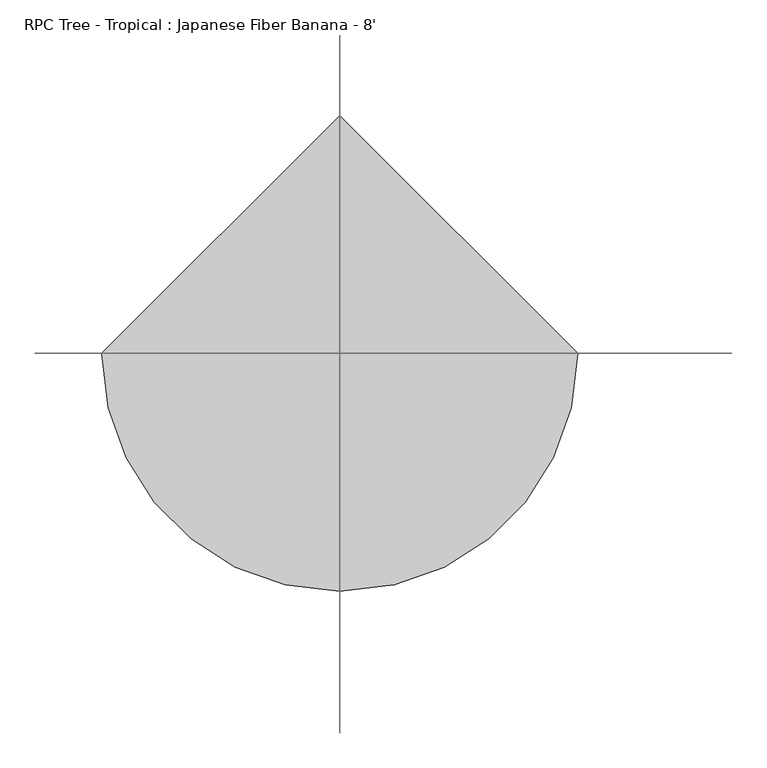
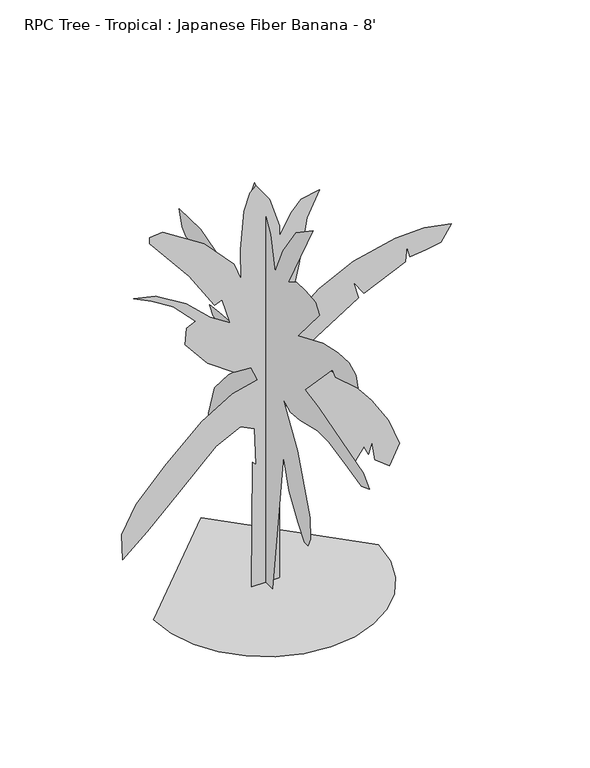
"""IFC4 building model written with IfcOpenShell, lengths in millimetres: geographic element geometry, RPC Tree - Tropical : Japanese Fiber Banana - 8'."""

from ifc_helpers import new_model, si_unit, origin, place, context, project, spatial, triangles, source, transform, mapped, element, save


def rpc_tree_tropical_japanese_fiber_banana_8_fc2fb2a9(model_context):
    return source(origin(), model_context, "Body", "Tessellation", [
        triangles([(-649.7467501, 0.0, 3.7e-06), (-632.5712723, -148.8792756, 3.7e-06), (-583.6506755, -285.6010629, 3.7e-06), (-506.9043426, -406.2488949, 3.7e-06), (-406.2488949, -506.9043426, 3.7e-06), (-285.6010629, -583.6506755, 3.7e-06), (-148.8792756, -632.5712723, 3.7e-06), (2.84e-05, -649.7467501, 3.7e-06), (148.8792756, -632.5712723, 3.7e-06), (285.6010629, -583.6506755, 3.7e-06), (406.2488949, -506.9043426, 3.7e-06), (506.9043426, -406.2488949, 3.7e-06), (583.6506755, -285.6010629, 3.7e-06), (632.5712723, -148.8790212, 3.7e-06), (649.7467501, 5.68e-05, 3.7e-06), (-8.52e-05, 649.7467501, 3.7e-06), (73.5169788, -2.4e-06, 1488.9400761), (86.1999983, -4e-06, 1501.9626823), (108.3956093, -6.3e-06, 1521.7797867), (138.5178168, -9.4e-06, 1547.2586094), (174.9816703, -1.3e-05, 1577.2688416), (216.2016834, -1.69e-05, 1610.6750874), (260.5921424, -2.12e-05, 1646.3444218), (306.5688237, -2.56e-05, 1683.149152), (505.0933339, -3.74e-05, 1782.4125698), (746.7776007, -4.41e-05, 1838.5162674), (915.0912369, -4.46e-05, 1842.831847), (1070.4584976, -4.1e-05, 1812.6209003), (1010.0392931, -3.02e-05, 1721.9908218), (923.7222507, -2.81e-05, 1704.7264687), (833.0921722, -2.71e-05, 1696.0954548), (815.8277464, -3.48e-05, 1760.832637), (807.1968052, -2.45e-05, 1674.5181381), (565.5150455, -1.17e-05, 1566.6237064), (505.0933339, -2.2e-05, 1652.9382053), (535.3041716, -9.6e-06, 1549.3592079), (250.4636001, 1.15e-05, 1372.4146305), (207.3058056, 2.02e-05, 1299.0465797), (457.6205775, 4.54e-05, 1087.573078), (608.672295, 6.81e-05, 897.679509), (707.9358582, 8.66e-05, 742.3123209), (772.6704969, 0.0001061, 578.3115755), (712.2512924, 0.00012, 461.7861663), (630.2496843, 0.0001123, 526.5233485), (612.9878019, 9.89e-05, 638.7333235), (591.4078691, 0.0001066, 573.9961049), (565.5150455, 0.0001, 630.1023823), (518.0422892, 0.0001082, 561.0496931), (237.5161527, 6.86e-05, 893.3640747), (99.411601, 4.9e-05, 1057.362204), (82.1486921, 4.08e-05, 1126.4148932), (77.8327038, 0.0001751, 0.0), (-81.8504909, 0.0001751, 0.0), (-77.5347659, 8.45e-05, 759.5742033), (-55.9558732, 8.71e-05, 737.996814), (-64.587582, 6.09e-05, 958.1012569), (-146.5871735, 5.57e-05, 1001.2585064), (-289.0071958, 6.39e-05, 932.2058172), (-500.4806794, 8.86e-05, 725.0478951), (-686.0587051, 0.0001097, 548.1032813), (-828.4769743, 0.0001241, 427.259858), (-832.7950247, 0.0001056, 582.6295896), (-750.7934166, 8.71e-05, 737.996814), (-573.8488029, 6.5e-05, 923.574876), (-371.0062786, 4.28e-05, 1109.1529381), (-194.0604295, 3e-05, 1217.044899), (-47.3244142, 2.59e-05, 1251.5712799), (-86.1662158, 1.56e-05, 1337.8882496), (-185.4289796, 1.46e-05, 1346.5192635), (-336.4799704, 1.7e-06, 1454.4136951), (-465.9543348, -1.73e-05, 1614.0963902), (-457.3233936, -2.87e-05, 1709.0419029), (-405.5326232, -3.18e-05, 1734.93727), (-535.0069877, -4.77e-05, 1868.7272141), (-660.1633381, -5.7e-05, 1946.4106991), (-763.7423355, -6.31e-05, 1998.1989624), (-638.583478, -5.95e-05, 1967.9881611), (-461.6388642, -4.67e-05, 1860.0962002), (-323.5335222, -3.12e-05, 1730.6218357), (-207.0078768, -2.25e-05, 1657.2536396), (-254.4808694, -4.1e-05, 1812.6209003), (-297.6381552, -3.9e-05, 1795.3590179), (-444.3744384, -6.62e-05, 2024.0943295), (-673.1097862, -9.91e-05, 2300.30247), (-673.1097862, -0.0001038, 2339.1442852), (-595.4261559, -0.0001043, 2343.4597195), (-358.0598668, -8.63e-05, 2192.4080383), (-185.4289796, -6.42e-05, 2006.8299763), (-142.2711851, -5.13e-05, 1898.9380154), (-146.5871735, -7.29e-05, 2080.198027), (-125.0082762, -0.0001002, 2308.9359547), (-90.4819498, -0.000112, 2408.1969017), (-55.9558732, -0.0001156, 2438.4078484), (21.7278389, -0.0001027, 2330.5132713), (77.8327038, -8.11e-05, 2149.2507889), (77.8327038, -7.39e-05, 2088.8315117), (146.8851113, -8.78e-05, 2205.3569572), (202.9900806, -9.5e-05, 2265.7760891), (310.8842943, -9.76e-05, 2287.3560219), (237.5161527, -8.01e-05, 2140.619775), (190.0426515, -4.87e-05, 1877.3580826), (142.5693864, -2.3e-05, 1661.5692192), (124.24932, -1.81e-05, 1620.2990639), (106.9864112, -1.34e-05, 1581.1042179), (91.8370452, -9.2e-06, 1546.0623161), (79.8586157, -5.8e-06, 1517.2485226), (72.1077807, -3.4e-06, 1496.740472), (69.6416885, -2.1e-06, 1486.6108578), (-6.07e-05, -228.3904198, 1972.5652073), (-6.46e-05, -305.2429235, 2016.4820034), (-6.49e-05, -396.7365758, 2020.139629), (-6.39e-05, -495.5454429, 2009.1616653), (-5.9e-05, -535.8019973, 1954.2670509), (-3.61e-05, -319.883527, 1698.0893738), (-4.56e-05, -568.7408298, 1804.2211224), (-4.86e-05, -718.786722, 1837.1573387), (-4.89e-05, -828.5760235, 1840.8175804), (-4.63e-05, -901.771483, 1811.5388443), (-4.01e-05, -920.0697121, 1742.0061699), (-3.38e-05, -696.8283966, 1672.4708794), (-3.65e-05, -667.5522039, 1701.7496155), (-1.06e-05, -393.0764068, 1412.635722), (-8.3e-06, -524.8241063, 1387.0172276), (3.5e-06, -974.9643265, 1255.2694553), (8.7e-06, -1037.1792789, 1196.7146719), (1.13e-05, -956.6660975, 1167.4360085), (8.7e-06, -821.2583015, 1196.7146719), (5.1e-06, -623.6354805, 1236.971299), (5.1e-06, -517.5038046, 1236.971299), (8.7e-06, -341.8393816, 1196.7146719), (9.7e-06, -246.688885, 1185.7342375), (6.4e-06, -169.8356182, 1222.3306229), (2.67e-05, -316.2233943, 995.4317545), (5.65e-05, -440.6507558, 662.4010649), (6.79e-05, -447.9710575, 534.3135707), (7.28e-05, -422.3525631, 479.4163765), (7.28e-05, -385.756105, 479.4163765), (6.53e-05, -323.5411526, 563.5896907), (5.32e-05, -232.0500619, 698.9975229), (3.75e-05, -177.1549025, 874.6619459), (5.84e-05, -147.8774926, 640.4427395), (0.0001157, -67.36457, 3.7e-06), (0.0001157, 82.6820898, 3.7e-06), (9.61e-05, 82.6820898, 219.5804016), (0.0001026, 64.3836201, 146.3870222), (7.84e-05, 35.1062147, 417.2039675), (4.99e-05, 35.1062147, 735.593981), (2.38e-05, 79.0221933, 1028.3680435), (2.8e-05, 174.1739435, 980.7936945), (4.14e-05, 331.5396469, 830.7452225), (5.19e-05, 430.3510211, 713.6355829), (5.84e-05, 444.9891174, 640.4427395), (5.58e-05, 470.6076118, 669.7214029), (6.33e-05, 466.9474792, 585.5480887), (6.01e-05, 529.1624316, 622.1445105), (6.5e-05, 551.1207933, 567.2498597), (5.45e-05, 573.0791914, 684.3594629), (3.75e-05, 514.5243716, 874.6619459), (2.28e-05, 375.4563704, 1039.3484779), (6.1e-06, 170.5143013, 1225.9908646), (1.8e-06, 272.9848271, 1273.567757), (-1.1e-06, 393.7545994, 1306.5039734), (2e-07, 459.6297209, 1291.8659134), (-1.1e-06, 529.1624316, 1306.5039734), (-5e-06, 565.7588533, 1350.4207695), (-6.4e-06, 466.9474792, 1365.0588295), (-7.7e-06, 254.6866163, 1379.6968895), (-1.32e-05, 331.5396469, 1441.911842), (-2.5e-05, 514.5243716, 1573.6594688), (-2.96e-05, 730.4453854, 1624.896603), (-2.96e-05, 799.9781324, 1624.896603), (-3.29e-05, 840.2346869, 1661.4929157), (-4.1e-05, 869.5133503, 1752.9841335), (-4.14e-05, 653.5923729, 1756.6442299), (-3.58e-05, 441.3289484, 1694.4292774), (-3.02e-05, 283.9652797, 1632.214325), (-1.62e-05, 108.2998484, 1474.8480583), (-5.35e-05, 152.215827, 1892.0520985), (-8.06e-05, 185.15287, 2195.804052), (-9.63e-05, 111.9594906, 2371.468475), (-9.01e-05, 46.0854001, 2301.9356552), (-7.67e-05, -45.4067079, 2151.889872), (-5.87e-05, -89.322691, 1950.6068092), (-7.44e-05, -169.8356182, 2126.2712322), (-9.14e-05, -301.5827909, 2316.5737152), (-0.0001016, -469.9294556, 2430.0231857)], [[15, 16, 1], [14, 15, 1], [14, 1, 2], [13, 14, 2], [13, 2, 3], [13, 3, 4], [12, 13, 4], [11, 12, 4], [11, 4, 5], [11, 5, 6], [11, 6, 7], [11, 7, 8], [11, 8, 9], [11, 9, 10], [75, 76, 77], [45, 46, 47], [53, 54, 55], [60, 61, 62], [98, 99, 100], [97, 98, 100], [27, 28, 29], [27, 29, 30], [47, 48, 49], [60, 62, 63], [59, 60, 63], [59, 63, 64], [58, 59, 64], [58, 64, 65], [74, 75, 77], [74, 77, 78], [73, 74, 78], [73, 78, 79], [42, 43, 44], [42, 44, 45], [41, 42, 45], [92, 93, 94], [91, 92, 94], [96, 97, 100], [96, 100, 101], [52, 53, 55], [51, 52, 55], [51, 55, 56], [57, 58, 65], [57, 65, 66], [57, 66, 67], [27, 30, 31], [27, 31, 32], [26, 27, 32], [84, 85, 86], [83, 84, 86], [83, 86, 87], [83, 87, 88], [82, 83, 88], [81, 82, 88], [81, 88, 89], [56, 57, 67], [51, 56, 67], [91, 94, 95], [90, 91, 95], [90, 95, 96], [89, 90, 96], [89, 96, 101], [89, 101, 102], [33, 34, 35], [32, 33, 35], [26, 32, 35], [25, 26, 35], [24, 25, 35], [81, 89, 102], [80, 81, 102], [80, 102, 103], [80, 103, 104], [80, 104, 105], [80, 105, 106], [80, 106, 107], [40, 41, 45], [40, 45, 47], [40, 47, 49], [39, 40, 49], [38, 39, 49], [38, 49, 50], [38, 50, 51], [38, 51, 67], [38, 67, 68], [35, 36, 37], [24, 35, 37], [23, 24, 37], [22, 23, 37], [21, 22, 37], [20, 21, 37], [19, 20, 37], [18, 19, 37], [17, 18, 37], [17, 37, 38], [17, 38, 68], [108, 17, 68], [80, 107, 108], [80, 108, 68], [80, 68, 69], [80, 69, 70], [80, 70, 71], [79, 80, 71], [73, 79, 71], [73, 71, 72], [143, 144, 145], [185, 186, 109], [184, 185, 109], [155, 156, 157], [183, 184, 109], [151, 152, 153], [153, 154, 155], [164, 165, 166], [163, 164, 166], [124, 125, 126], [179, 180, 181], [172, 173, 174], [171, 172, 174], [170, 171, 174], [169, 170, 174], [169, 174, 175], [142, 143, 145], [141, 142, 145], [141, 145, 146], [141, 146, 147], [140, 141, 147], [140, 147, 148], [162, 163, 166], [162, 166, 167], [161, 162, 167], [179, 181, 182], [178, 179, 182], [178, 182, 183], [153, 155, 157], [153, 157, 158], [151, 153, 158], [150, 151, 158], [150, 158, 159], [149, 150, 159], [149, 159, 160], [148, 149, 160], [124, 126, 127], [123, 124, 127], [123, 127, 128], [123, 128, 129], [118, 119, 120], [117, 118, 120], [116, 117, 120], [116, 120, 121], [115, 116, 121], [115, 121, 122], [114, 115, 122], [168, 169, 175], [168, 175, 176], [168, 176, 177], [167, 168, 177], [177, 178, 183], [122, 123, 129], [122, 129, 130], [112, 113, 114], [111, 112, 114], [110, 111, 114], [109, 110, 114], [183, 109, 114], [177, 183, 114], [177, 114, 122], [177, 122, 130], [177, 130, 131], [177, 131, 132], [167, 177, 132], [161, 167, 132], [160, 161, 132], [148, 160, 132], [140, 148, 132], [140, 132, 133], [140, 133, 134], [139, 140, 134], [138, 139, 134], [138, 134, 135], [137, 138, 135], [137, 135, 136]], closed=False),
    ])


if __name__ == "__main__":
    model = new_model("IFC4")
    model_context = context("Model", 3, world=origin())
    ifc_project = project(units=[si_unit("LENGTHUNIT", "METRE", prefix="MILLI")], contexts=[model_context])
    site = spatial("IfcSite", under=ifc_project)
    building = spatial("IfcBuilding", under=site)
    placement = place(None, origin())
    rpc_tree_tropical_japanese_fiber_banana_8_shape = rpc_tree_tropical_japanese_fiber_banana_8_fc2fb2a9(model_context)
    element("IfcGeographicElement", 1, ObjectType="RPC Tree - Tropical : Japanese Fiber Banana - 8'", at=placement, inside=building, context=model_context, shape_type="MappedRepresentation", body=[
        mapped(rpc_tree_tropical_japanese_fiber_banana_8_shape, transform((0.0, 0.0, 0.0), x_axis=(1.0, 0.0, 0.0), y_axis=(0.0, 1.0, 0.0), z_axis=(0.0, 0.0, 1.0))),
    ])
    save(model, "model.ifc")

# Revit data of these elements
# Type "RPC Tree - Tropical : Japanese Fiber Banana - 8'"
#   built-in parameter 1005198 = "{2, 15},{39, RPC-16-FVGT-NR7X-7G1M-A000-ST1L-LVER-AU},{1, 0},{1, 0},{2, 13},{1, 8},{5, Color},{1, 0},{1, 0},{3, 0.8},{3, 0.8},{3, 0.8},{1, 8},{7, BBoxMin},{1, 0},{1, 0},{1, 0},{1, 0},{1, 0},{1, 8},{7, BBoxMax},{1, 0},{1, 0},{1, 0},{1, 0},{1, 0},{2, 11},{9, RPCTypeId},{1, 0},{1, 0},{39, RPC-16-FVGT-NR7X-7G1M-A000-ST1L-LVER-AU},{1, 6},{14, RPCPlantHeight},{1, 0},{1, 0},{1, 8},{2, 11},{7, keyword},{1, 0},{1, 0},{35, :RPCs:Trees [Tropical]:Geometry:RPC},{2, 11},{8, category},{1, 0},{1, 0},{16, Trees [Tropical]},{2, 11},{12, LocalizedUID},{1, 0},{1, 0},{21, Japanese Fiber Banana},{2, 14},{6, Height},{1, 0},{1, 0},{1, 8},{1, 2},{16, Cast Reflections},{1, 0},{1, 0},{1, 0},{1, 2},{12, Cast Shadows},{1, 0},{1, 0},{1, 1},{1, 2},{9, Lock View},{1, 0},{1, 0},{1, 0},{1, 4},{5, ViewC},{1, 0},{1, 0},{1, 0},{21, assetlibrary_base.fbx},{1, 5},"
#   built-in parameter 1005195 = "RPC-16-FVGT-NR7X-7G1M-A000-ST1L-LVER-AU"
#   Type Comments = "Japanese Fiber Banana"
#   Assembly Code = "G2050500"
#   Height = 8' - 0"
#   Plan Symbol = element 361270
#   Default Elevation = 0
